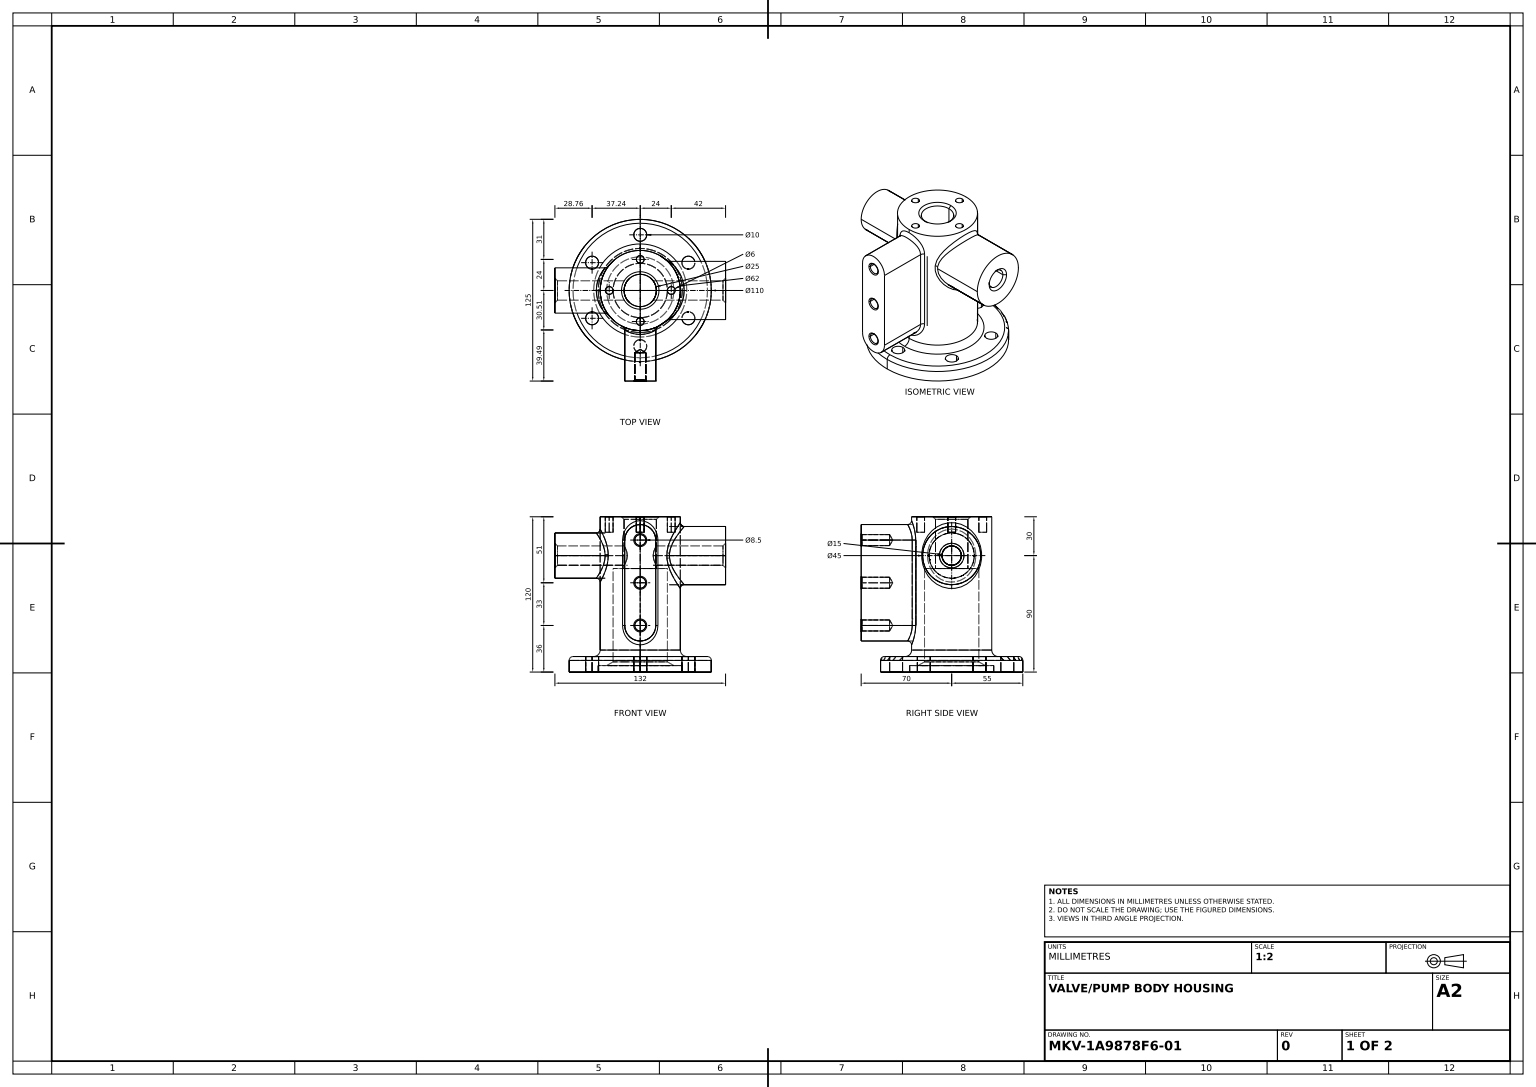
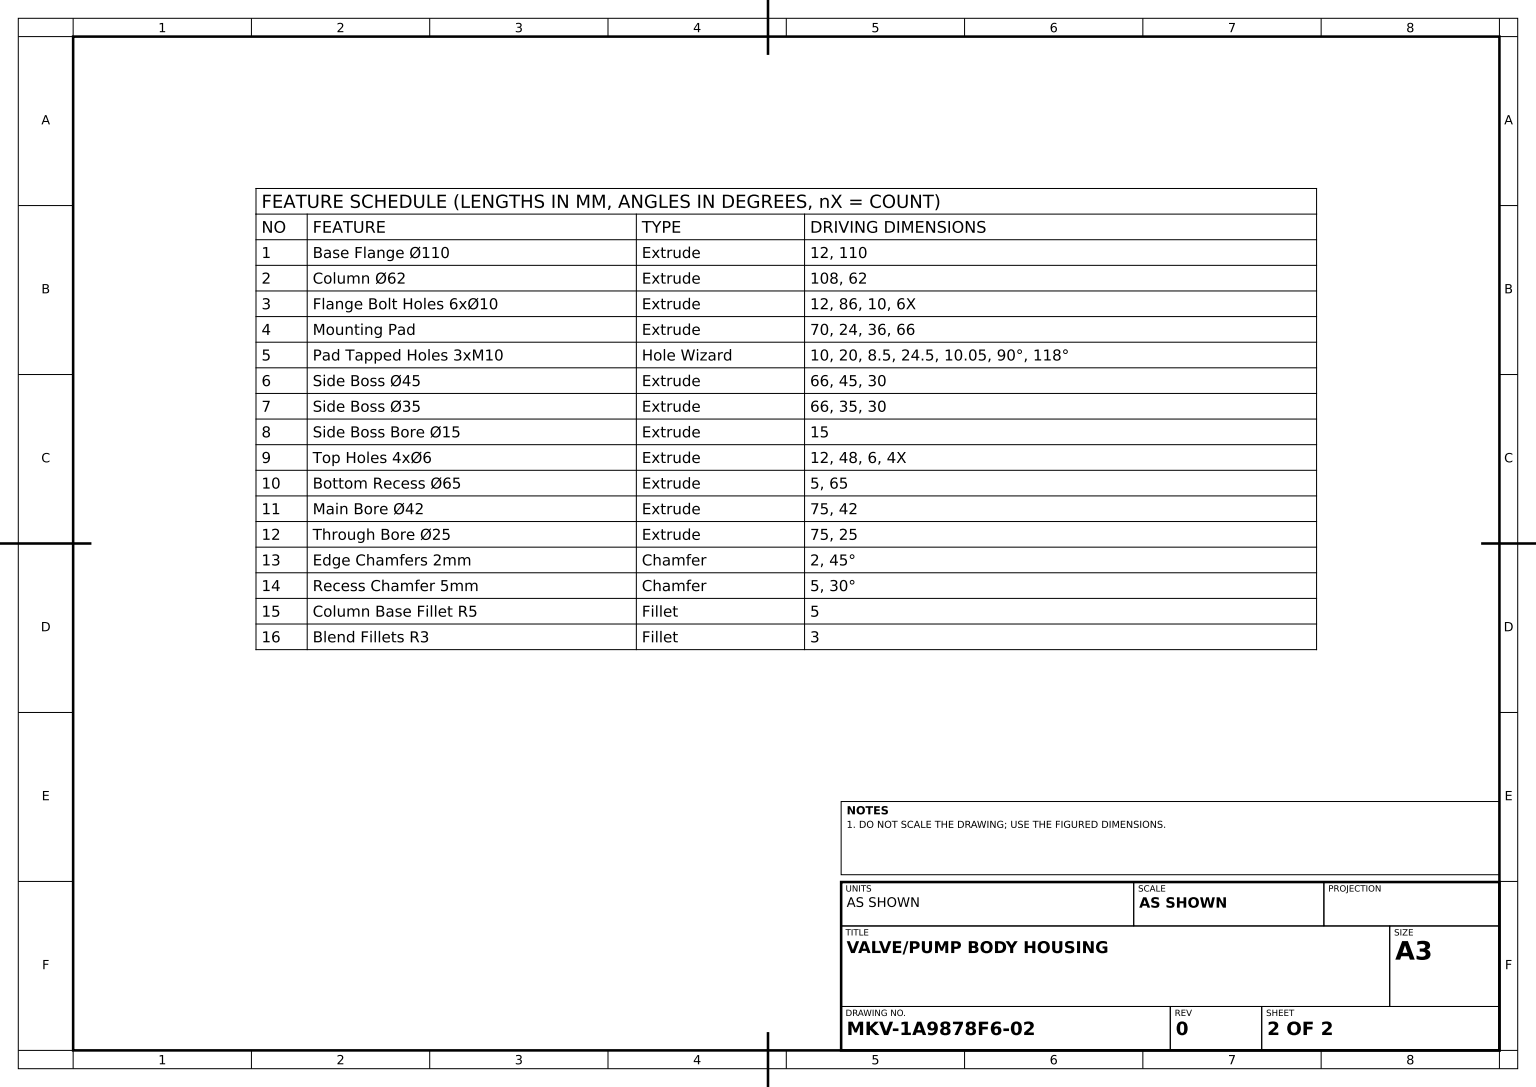
from build123d import *

# Parameters (mm, degrees)
BASE_FLANGE_SKETCH_R               = 55
BASE_FLANGE_110_DEPTH              = 12
COLUMN_SKETCH_R                    = 31
COLUMN_62_DEPTH                    = 108
FLANGE_BOLT_HOLES_SKETCH_R         = 5
FLANGE_BOLT_HOLES_6X_10_DEPTH      = 12
MOUNTING_PAD_REACH                 = 183.797
MOUNTING_PAD_END_RADIUS            = 31
PAD_TAPPED_HOLES_3XM10_D           = 8.5
PAD_TAPPED_HOLES_3XM10_DEPTH       = 21.946342369
PAD_TAPPED_HOLES_3XM10_CSINK_D     = 10.05
PAD_TAPPED_HOLES_3XM10_CSINK_ANGLE = 90
PAD_TAPPED_HOLES_3XM10_TIP         = 2.553657631
SIDE_BOSS_45_REACH                 = 186.231
SIDE_BOSS_45_END_RADIUS            = 31
SIDE_BOSS_45_SKETCH_R              = 22.5
SIDE_BOSS_35_REACH                 = 193.635
SIDE_BOSS_35_END_RADIUS            = 31
SIDE_BOSS_35_SKETCH_R              = 17.5
SIDE_BOSS_BORE_SKETCH_R            = 7.5
SIDE_BOSS_BORE_15_DEPTH            = 192.635070027
TOP_HOLES_SKETCH_R                 = 3
TOP_HOLES_4X_6_DEPTH               = 12
BOTTOM_RECESS_SKETCH_R             = 32.5
BOTTOM_RECESS_65_DEPTH             = 5
MAIN_BORE_SKETCH_R                 = 21
MAIN_BORE_42_DEPTH                 = 75
THROUGH_BORE_SKETCH_R              = 12.5
THROUGH_BORE_25_DEPTH              = 75
EDGE_CHAMFERS_2MM_SIZE             = 2
RECESS_CHAMFER_5MM_SIZE            = 5
RECESS_CHAMFER_5MM_SIZE2           = 2.886751346
COLUMN_BASE_FILLET_R5_R            = 5
BLEND_FILLETS_R3_R                 = 3


with BuildPart() as part:
    # Base Flange Sketch → Base Flange Ø110 (new body)
    with BuildSketch(Plane(origin=(0, 0, 0), x_dir=(1, 0, 0), z_dir=(0, 1, 0))):
        with Locations(Location((0, 0, 0), (0, 0, 270))):
            Circle(BASE_FLANGE_SKETCH_R)
    extrude(amount=BASE_FLANGE_110_DEPTH)

    # Column Sketch → Column Ø62 (add)
    with BuildSketch(Plane(origin=(0, 12, 0), x_dir=(1, 0, 0), z_dir=(0, 1, 0))):
        with Locations(Location((0, 0, 0), (0, 0, 270))):
            Circle(COLUMN_SKETCH_R)
    extrude(amount=COLUMN_62_DEPTH)

    # Flange Bolt Holes Sketch → Flange Bolt Holes 6xØ10 (cut)
    with BuildSketch(Plane(origin=(0, 12, 0), x_dir=(1, 0, 0), z_dir=(0, 1, 0))):
        with Locations(Location((0, 43, 0), (0, 0, 270))):
            Circle(FLANGE_BOLT_HOLES_SKETCH_R)
        with Locations(Location((37.239092363, 21.5, 0), (0, 0, 270))):
            Circle(FLANGE_BOLT_HOLES_SKETCH_R)
        with Locations(Location((37.239092363, -21.5, 0), (0, 0, 270))):
            Circle(FLANGE_BOLT_HOLES_SKETCH_R)
        with Locations(Location((0, -43, 0), (0, 0, 270))):
            Circle(FLANGE_BOLT_HOLES_SKETCH_R)
        with Locations(Location((-37.239092363, -21.5, 0), (0, 0, 270))):
            Circle(FLANGE_BOLT_HOLES_SKETCH_R)
        with Locations(Location((-37.239092363, 21.5, 0), (0, 0, 270))):
            Circle(FLANGE_BOLT_HOLES_SKETCH_R)
    extrude(amount=-FLANGE_BOLT_HOLES_6X_10_DEPTH, mode=Mode.SUBTRACT)

    # Mounting Pad: up to this cylinder (the profile starts outside it)
    mounting_pad_end = Plane(origin=(0, 69, 0), z_dir=(0, -1, 0)) * Cylinder(MOUNTING_PAD_END_RADIUS, 430.594, mode=Mode.PRIVATE)
    # Mounting Pad Sketch → Mounting Pad (add, up to the surface)
    with BuildSketch(Plane.XY.offset(70), mode=Mode.PRIVATE) as mounting_pad_sk1:
        with BuildLine():
            Line((-12, 102), (-12, 36))
            ThreePointArc((-12, 36), (0, 24), (12, 36))
            Line((12, 36), (12, 102))
            ThreePointArc((12, 102), (0, 114), (-12, 102))
        make_face()
    mounting_pad_tool1 = extrude(mounting_pad_sk1.sketch, amount=-MOUNTING_PAD_REACH, mode=Mode.PRIVATE) - mounting_pad_end
    add(mounting_pad_tool1.solids().sort_by_distance((0, 69, 70))[0])

    # Pad Tapped Holes 3xM10
    with Locations(Plane.XY.offset(70)):
        with Locations((0, 102), (0, 69), (0, 36)):
            CounterSinkHole(PAD_TAPPED_HOLES_3XM10_D / 2, PAD_TAPPED_HOLES_3XM10_CSINK_D / 2, depth=PAD_TAPPED_HOLES_3XM10_DEPTH, counter_sink_angle=PAD_TAPPED_HOLES_3XM10_CSINK_ANGLE)
            with Locations((0, 0, -(PAD_TAPPED_HOLES_3XM10_DEPTH + PAD_TAPPED_HOLES_3XM10_TIP / 2))):  # 118° drill point
                Cone(0, PAD_TAPPED_HOLES_3XM10_D / 2, PAD_TAPPED_HOLES_3XM10_TIP, mode=Mode.SUBTRACT)

    # Side Boss Ø45: up to this cylinder (the profile starts outside it)
    side_boss_45_end = Plane(origin=(0, 90, 0), z_dir=(0, -1, 0)) * Cylinder(SIDE_BOSS_45_END_RADIUS, 435.462, mode=Mode.PRIVATE)
    # Side Boss Ø45 Sketch → Side Boss Ø45 (add, up to the surface)
    with BuildSketch(Plane(origin=(66, 0, 0), x_dir=(0, 0, -1), z_dir=(1, 0, 0)), mode=Mode.PRIVATE) as side_boss_45_sk1:
        with Locations((0, 90)):
            Circle(SIDE_BOSS_45_SKETCH_R)
    side_boss_45_tool1 = extrude(side_boss_45_sk1.sketch, amount=-SIDE_BOSS_45_REACH, mode=Mode.PRIVATE) - side_boss_45_end
    add(side_boss_45_tool1.solids().sort_by_distance((66, 90, 0))[0])

    # Side Boss Ø35: up to this cylinder (the profile starts outside it)
    side_boss_35_end = Plane(origin=(0, 90, 0), z_dir=(0, -1, 0)) * Cylinder(SIDE_BOSS_35_END_RADIUS, 450.27, mode=Mode.PRIVATE)
    # Side Boss Ø35 Sketch → Side Boss Ø35 (add, up to the surface)
    with BuildSketch(Plane(origin=(-66, 0, 0), x_dir=(0, 0, -1), z_dir=(1, 0, 0)), mode=Mode.PRIVATE) as side_boss_35_sk1:
        with Locations(Location((0, 90, 0), (0, 0, 180))):
            Circle(SIDE_BOSS_35_SKETCH_R)
    side_boss_35_tool1 = extrude(side_boss_35_sk1.sketch, amount=SIDE_BOSS_35_REACH, mode=Mode.PRIVATE) - side_boss_35_end
    add(side_boss_35_tool1.solids().sort_by_distance((-66, 90, 0))[0])

    # Side Boss Bore Sketch → Side Boss Bore Ø15 (cut, through all)
    with BuildSketch(Plane(origin=(66, 0, 0), x_dir=(0, 0, -1), z_dir=(1, 0, 0))):
        with Locations((0, 90)):
            Circle(SIDE_BOSS_BORE_SKETCH_R)
    extrude(amount=-SIDE_BOSS_BORE_15_DEPTH, mode=Mode.SUBTRACT)

    # Top Holes Sketch → Top Holes 4xØ6 (cut)
    with BuildSketch(Plane(origin=(0, 120, 0), x_dir=(1, 0, 0), z_dir=(0, 1, 0))):
        with Locations(Location((0, 24, 0), (0, 0, 270))):
            Circle(TOP_HOLES_SKETCH_R)
        with Locations(Location((24, 0, 0), (0, 0, 270))):
            Circle(TOP_HOLES_SKETCH_R)
        with Locations(Location((0, -24, 0), (0, 0, 270))):
            Circle(TOP_HOLES_SKETCH_R)
        with Locations(Location((-24, 0, 0), (0, 0, 270))):
            Circle(TOP_HOLES_SKETCH_R)
    extrude(amount=-TOP_HOLES_4X_6_DEPTH, mode=Mode.SUBTRACT)

    # Bottom Recess Sketch → Bottom Recess Ø65 (cut)
    with BuildSketch(Plane.XZ):
        with Locations(Location((0, 0, 0), (0, 0, 270))):
            Circle(BOTTOM_RECESS_SKETCH_R)
    extrude(amount=-BOTTOM_RECESS_65_DEPTH, mode=Mode.SUBTRACT)

    # Main Bore Sketch → Main Bore Ø42 (cut)
    with BuildSketch(Plane.XZ.offset(-5)):
        with Locations(Location((0, 0, 0), (0, 0, 270))):
            Circle(MAIN_BORE_SKETCH_R)
    extrude(amount=-MAIN_BORE_42_DEPTH, mode=Mode.SUBTRACT)

    # Through Bore Sketch → Through Bore Ø25 (cut)
    with BuildSketch(Plane.XZ.offset(-80)):
        with Locations(Location((0, 0, 0), (0, 0, 270))):
            Circle(THROUGH_BORE_SKETCH_R)
    extrude(amount=-THROUGH_BORE_25_DEPTH, mode=Mode.SUBTRACT)

    # Edge Chamfers 2mm
    edge_chamfers_2mm_edges = [part.edges().sort_by_distance(p)[0] for p in [
        (0, 120, 12.5),
        (-66, 90, 7.5),
        (66, 90, 7.5),
    ]]
    chamfer(edge_chamfers_2mm_edges, length=EDGE_CHAMFERS_2MM_SIZE)

    # Recess Chamfer 5mm
    recess_chamfer_5mm_edges = [part.edges().sort_by_distance(p)[0] for p in [
        (0, 5, 21),
    ]]
    recess_chamfer_5mm_side = [part.faces().sort_by_distance(p)[0] for p in [
        (0, 5, 31.580761184),
    ]]
    chamfer(recess_chamfer_5mm_edges, length=RECESS_CHAMFER_5MM_SIZE, length2=RECESS_CHAMFER_5MM_SIZE2, reference=recess_chamfer_5mm_side[0])

    # Column Base Fillet R5
    column_base_fillet_r5_edges = [part.edges().sort_by_distance(p)[0] for p in [
        (0, 12, -31),
    ]]
    fillet(column_base_fillet_r5_edges, radius=COLUMN_BASE_FILLET_R5_R)

    # Blend Fillets R3
    blend_fillets_r3_edges = [part.edges().sort_by_distance(p)[0] for p in [
        (-8.487533434, 110.483028718, 29.815462033),
        (-12, 69, 28.583211856),
        (8.487533434, 27.516971282, 29.815462033),
        (12, 69, 28.583211856),
        (0, 12, -55),
        (21.324868112, 90, 22.5),
        (-25.588083164, 90, -17.5),
    ]]
    fillet(blend_fillets_r3_edges, radius=BLEND_FILLETS_R3_R)


solid = part.part
